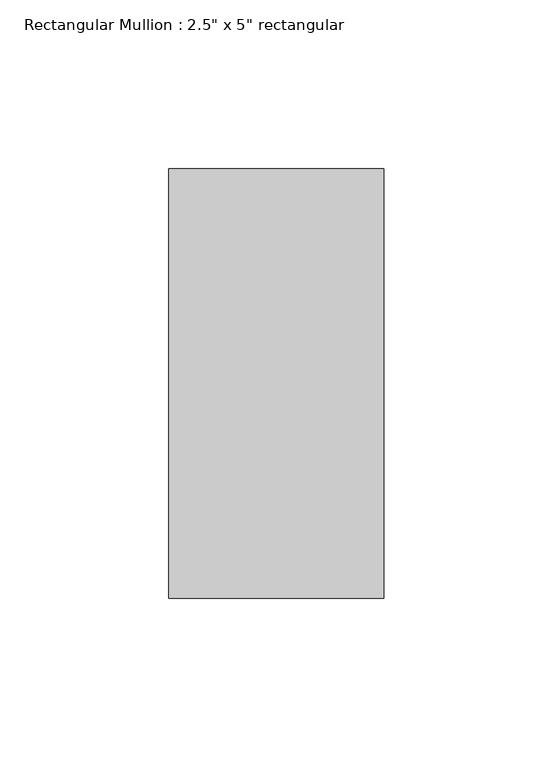
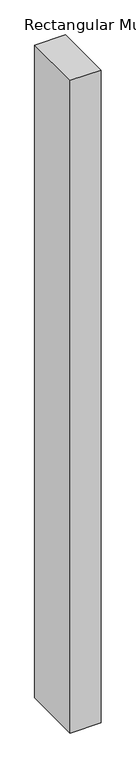
"""IFC4 building model written with IfcOpenShell, lengths in millimetres: member geometry."""

from ifc_helpers import new_model, si_unit, frame, origin, place, context, project, spatial, polyline, outline, extrude, source, transform, mapped, element, save


def member_9ad43860(model_context):
    return source(origin(), model_context, "Body", "SweptSolid", [
        extrude(outline(polyline([(0.0, 63.5), (0.0, -63.5), (-63.5, -63.5), (-63.5, 63.5), (0.0, 63.5)])), frame((0.0, 0.0, -1426.4677433), z_axis=(0.0, 0.0, 1.0), x_axis=(1.0, 0.0, 0.0)), (0.0, 0.0, 1.0), 1426.4677433),
    ])


if __name__ == "__main__":
    model = new_model("IFC4")
    model_context = context("Model", 3, world=origin())
    ifc_project = project(units=[si_unit("LENGTHUNIT", "METRE", prefix="MILLI")], contexts=[model_context])
    site = spatial("IfcSite", under=ifc_project)
    building = spatial("IfcBuilding", under=site)
    placement = place(None, origin())
    member_shape = member_9ad43860(model_context)
    element("IfcMember", 1, ObjectType="Rectangular Mullion : 2.5\" x 5\" rectangular", at=placement, inside=building, context=model_context, shape_type="MappedRepresentation", body=[
        mapped(member_shape, transform((0.0, 0.0, 0.0), x_axis=(1.0, 0.0, 0.0), y_axis=(0.0, 1.0, 0.0), z_axis=(0.0, 0.0, 1.0))),
    ])
    save(model, "model.ifc")

# Revit data of these elements
# Type "Rectangular Mullion : 2.5\" x 5\" rectangular"
#   built-in parameter 1007304 = 0.416667 (stored number, unit not read)
#   built-in parameter 1007301 = 0.104167 (stored number, unit not read)
#   built-in parameter 1007300 = 0.104167 (stored number, unit not read)
# Element 1 (IfcMember, "Rectangular Mullion : 2.5\" x 5\" rectangular")
#   Materials on its faces: "Iron, Ductile"
# Materials
#   "Iron, Ductile": class "Metal", colour RGB 0 0 0, transparency 0, Description = "Ductile cast iron", Cost = 0
